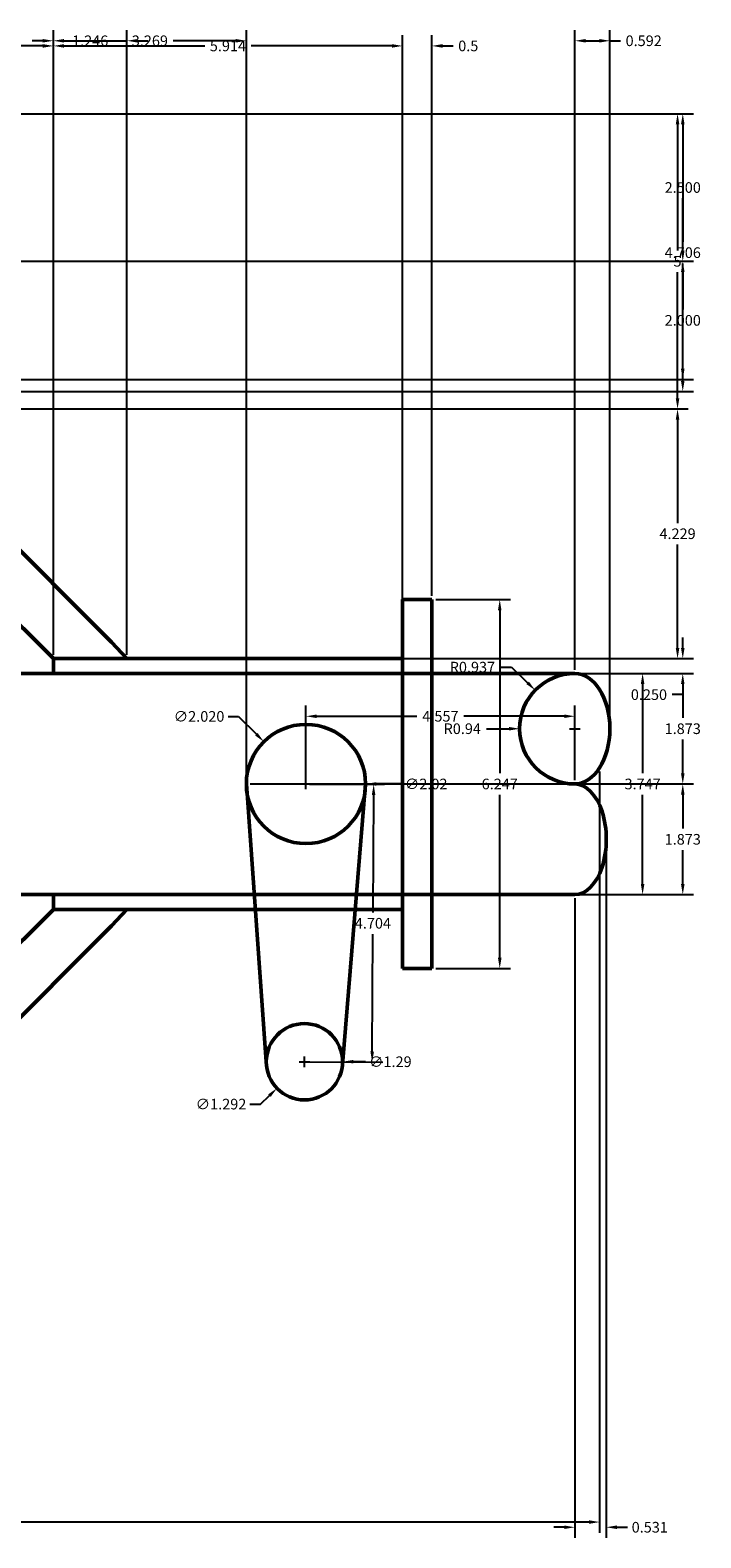
# Model space of a CAD drawing. Units: inches. Extents: x 15.4 to 41.1, y -0.4 to 25.1.
# Tile 4 of 4: x 29.7 to 41.1, y -0.4 to 25.1. Entities that reach past the tile are written whole.
import ezdxf

# ---------------------------------------------------------------- set-up
doc = ezdxf.new("R2010")
doc.units = ezdxf.units.IN
doc.header["$MEASUREMENT"] = 0
doc.layers.add('M-DIMS', color=2, linetype='Continuous', lineweight=18)
doc.layers.add('M-OUTL', color=7, linetype='Continuous', lineweight=50)
doc.styles.get("Standard").update_dxf_attribs({"font": 'arial.ttf'})
doc.dimstyles.get("Standard").update_dxf_attribs({"dimtxt": 0.18, "dimasz": 0.18, "dimexe": 0.18, "dimexo": 0.0625, "dimgap": 0.09, "dimtad": 0, "dimtih": 1, "dimtoh": 1, "dimdec": 4, "dimzin": 0, "dimdsep": 46, "dimtxsty": 'Standard', "dimcen": 0.09, "dimadec": 0, "dimazin": 0, "dimtfac": 1, "dimtdec": 4, "dimtofl": 0, "dimtmove": 0, "dimatfit": 3, "dimfxl": 1, "dimtolj": 1, "dimtzin": 0, "dimarcsym": 0})

# ---------------------------------------------------------------- blocks, each defined once
blk = doc.blocks.new('*D1')
at = {"layer": 'Defpoints', "color": 0, "transparency": 16777216}
for p in [(39.379, 12.649), (17.513, 10.885), (39.379, -0.125)]:
    blk.add_point(p, dxfattribs=at)
at = {"layer": 'M-DIMS', "color": 0, "lineweight": -2, "transparency": 16777216}
for p, q in [((39.379, 12.587), (39.379, -0.305)), ((17.513, 10.823), (17.513, -0.305)), ((17.693, -0.125), (27.98, -0.125)), ((39.199, -0.125), (28.912, -0.125))]:
    blk.add_line(p, q, dxfattribs=at)
at = {"layer": 'M-DIMS', "color": 0, "transparency": 16777216}
for points in [[(17.693, -0.095), (17.693, -0.155), (17.513, -0.125)], [(39.199, -0.095), (39.199, -0.155), (39.379, -0.125)]]:
    blk.add_solid(points, dxfattribs=at)
at = {"layer": 'M-DIMS', "color": 0, "transparency": 16777216, "insert": (28.446, -0.125), "char_height": 0.18, "attachment_point": 5}
blk.add_mtext('\\A1;21.865', dxfattribs=at)
blk = doc.blocks.new('*D8')
at = {"layer": 'Defpoints', "color": 0, "transparency": 16777216}
for p in [(30.124, 24.875), (26.868, 19.021), (30.124, 14.498)]:
    blk.add_point(p, dxfattribs=at)
at = {"layer": 'M-DIMS', "color": 0, "lineweight": -2, "transparency": 16777216}
for p, q in [((26.868, 19.083), (26.868, 25.055)), ((30.124, 14.561), (30.124, 25.055)), ((27.048, 24.875), (28.172, 24.875)), ((29.944, 24.875), (28.819, 24.875))]:
    blk.add_line(p, q, dxfattribs=at)
at = {"layer": 'M-DIMS', "color": 0, "transparency": 16777216}
for points in [[(27.048, 24.905), (27.048, 24.845), (26.868, 24.875)], [(29.944, 24.905), (29.944, 24.845), (30.124, 24.875)]]:
    blk.add_solid(points, dxfattribs=at)
at = {"layer": 'M-DIMS', "color": 0, "transparency": 16777216, "insert": (28.496, 24.875), "char_height": 0.18, "attachment_point": 5}
blk.add_mtext('\\A1;3.26', dxfattribs=at)
blk = doc.blocks.new('*D9')
at = {"layer": 'Defpoints', "color": 0, "transparency": 16777216}
for p in [(36.038, 24.875), (30.124, 14.498), (36.038, 14.498)]:
    blk.add_point(p, dxfattribs=at)
at = {"layer": 'M-DIMS', "color": 0, "lineweight": -2, "transparency": 16777216}
for p, q in [((30.124, 14.561), (30.124, 25.055)), ((36.038, 14.561), (36.038, 25.055)), ((30.304, 24.875), (32.688, 24.875)), ((35.858, 24.875), (33.474, 24.875))]:
    blk.add_line(p, q, dxfattribs=at)
at = {"layer": 'M-DIMS', "color": 0, "transparency": 16777216}
for points in [[(30.304, 24.905), (30.304, 24.845), (30.124, 24.875)], [(35.858, 24.905), (35.858, 24.845), (36.038, 24.875)]]:
    blk.add_solid(points, dxfattribs=at)
at = {"layer": 'M-DIMS', "color": 0, "transparency": 16777216, "insert": (33.081, 24.875), "char_height": 0.18, "attachment_point": 5}
blk.add_mtext('\\A1;5.914', dxfattribs=at)
blk = doc.blocks.new('*D10')
at = {"layer": 'Defpoints', "color": 0, "transparency": 16777216}
for p in [(36.538, 24.875), (36.038, 15.498), (36.538, 15.498)]:
    blk.add_point(p, dxfattribs=at)
at = {"layer": 'M-DIMS', "color": 0, "lineweight": -2, "transparency": 16777216}
for p, q in [((36.038, 15.561), (36.038, 25.055)), ((36.538, 15.561), (36.538, 25.055)), ((35.858, 24.875), (35.678, 24.875)), ((36.718, 24.875), (36.898, 24.875))]:
    blk.add_line(p, q, dxfattribs=at)
at = {"layer": 'M-DIMS', "color": 0, "transparency": 16777216}
for points in [[(35.858, 24.905), (35.858, 24.845), (36.038, 24.875)], [(36.718, 24.905), (36.718, 24.845), (36.538, 24.875)]]:
    blk.add_solid(points, dxfattribs=at)
at = {"layer": 'M-DIMS', "color": 0, "transparency": 16777216, "insert": (37.153, 24.875), "char_height": 0.18, "attachment_point": 5}
blk.add_mtext('\\A1;0.5', dxfattribs=at)
blk = doc.blocks.new('*D11')
at = {"layer": 'Defpoints', "color": 0, "transparency": 16777216}
for p in [(26.868, 23.727), (25.868, 18.727), (40.699, 18.727)]:
    blk.add_point(p, dxfattribs=at)
at = {"layer": 'M-DIMS', "color": 0, "lineweight": -2, "transparency": 16777216}
for p, q in [((26.93, 23.727), (40.879, 23.727)), ((40.699, 23.547), (40.699, 21.409)), ((40.699, 18.907), (40.699, 21.045)), ((25.93, 18.727), (40.879, 18.727))]:
    blk.add_line(p, q, dxfattribs=at)
at = {"layer": 'M-DIMS', "color": 0, "transparency": 16777216}
for points in [[(40.669, 23.547), (40.729, 23.547), (40.699, 23.727)], [(40.669, 18.907), (40.729, 18.907), (40.699, 18.727)]]:
    blk.add_solid(points, dxfattribs=at)
at = {"layer": 'M-DIMS', "color": 0, "transparency": 16777216, "insert": (40.699, 21.227), "char_height": 0.18, "attachment_point": 5}
blk.add_mtext('\\A1;5', dxfattribs=at)
blk = doc.blocks.new('*D12')
at = {"layer": 'Defpoints', "color": 0, "transparency": 16777216}
for p in [(25.868, 18.727), (30.124, 14.498), (40.699, 14.498)]:
    blk.add_point(p, dxfattribs=at)
at = {"layer": 'M-DIMS', "color": 0, "lineweight": -2, "transparency": 16777216}
for p, q in [((25.93, 18.727), (40.879, 18.727)), ((40.699, 18.547), (40.699, 16.794)), ((40.699, 14.678), (40.699, 16.431)), ((30.186, 14.498), (40.879, 14.498))]:
    blk.add_line(p, q, dxfattribs=at)
at = {"layer": 'M-DIMS', "color": 0, "transparency": 16777216}
for points in [[(40.669, 18.547), (40.729, 18.547), (40.699, 18.727)], [(40.669, 14.678), (40.729, 14.678), (40.699, 14.498)]]:
    blk.add_solid(points, dxfattribs=at)
at = {"layer": 'M-DIMS', "color": 0, "transparency": 16777216, "insert": (40.699, 16.613), "char_height": 0.18, "attachment_point": 5}
blk.add_mtext('\\A1;4.229', dxfattribs=at)
blk = doc.blocks.new('*D31')
at = {"layer": 'Defpoints', "color": 0, "transparency": 16777216}
for p in [(38.96, 14.248), (38.96, 10.501), (40.107, 10.501)]:
    blk.add_point(p, dxfattribs=at)
at = {"layer": 'M-DIMS', "color": 0, "lineweight": -2, "transparency": 16777216}
for p, q in [((39.022, 14.248), (40.287, 14.248)), ((40.107, 14.068), (40.107, 12.557)), ((40.107, 10.681), (40.107, 12.193)), ((39.022, 10.501), (40.287, 10.501))]:
    blk.add_line(p, q, dxfattribs=at)
at = {"layer": 'M-DIMS', "color": 0, "transparency": 16777216}
for points in [[(40.077, 14.068), (40.137, 14.068), (40.107, 14.248)], [(40.077, 10.681), (40.137, 10.681), (40.107, 10.501)]]:
    blk.add_solid(points, dxfattribs=at)
at = {"layer": 'M-DIMS', "color": 0, "transparency": 16777216, "insert": (40.107, 12.375), "char_height": 0.18, "attachment_point": 5}
blk.add_mtext('\\A1;3.747', dxfattribs=at)
blk = doc.blocks.new('*D32')
at = {"layer": 'Defpoints', "color": 0, "transparency": 16777216}
for p in [(36.538, 15.498), (36.538, 9.251), (37.686, 9.251)]:
    blk.add_point(p, dxfattribs=at)
at = {"layer": 'M-DIMS', "color": 0, "lineweight": -2, "transparency": 16777216}
for p, q in [((36.601, 15.498), (37.866, 15.498)), ((37.686, 15.318), (37.686, 12.557)), ((37.686, 9.431), (37.686, 12.193)), ((36.601, 9.251), (37.866, 9.251))]:
    blk.add_line(p, q, dxfattribs=at)
at = {"layer": 'M-DIMS', "color": 0, "transparency": 16777216}
for points in [[(37.656, 15.318), (37.716, 15.318), (37.686, 15.498)], [(37.656, 9.431), (37.716, 9.431), (37.686, 9.251)]]:
    blk.add_solid(points, dxfattribs=at)
at = {"layer": 'M-DIMS', "color": 0, "transparency": 16777216, "insert": (37.686, 12.375), "char_height": 0.18, "attachment_point": 5}
blk.add_mtext('\\A1;6.247', dxfattribs=at)
blk = doc.blocks.new('*D33')
at = {"layer": 'Defpoints', "color": 0, "transparency": 16777216}
for p in [(34.403, 12.375), (34.377, 7.671), (35.524, 7.664)]:
    blk.add_point(p, dxfattribs=at)
at = {"layer": 'M-DIMS', "color": 0, "lineweight": -2, "transparency": 16777216}
for p, q in [((34.465, 12.374), (35.73, 12.367)), ((35.549, 12.188), (35.538, 10.198)), ((35.525, 7.844), (35.536, 9.834)), ((34.439, 7.67), (35.704, 7.663))]:
    blk.add_line(p, q, dxfattribs=at)
at = {"layer": 'M-DIMS', "color": 0, "transparency": 16777216}
for points in [[(35.519, 12.189), (35.579, 12.188), (35.55, 12.368)], [(35.495, 7.845), (35.555, 7.844), (35.524, 7.664)]]:
    blk.add_solid(points, dxfattribs=at)
at = {"layer": 'M-DIMS', "color": 0, "transparency": 16777216, "insert": (35.537, 10.016), "char_height": 0.18, "attachment_point": 5}
blk.add_mtext('\\A1;4.704', dxfattribs=at)
blk = doc.blocks.new('*D34')
at = {"layer": 'Defpoints', "color": 0, "transparency": 16777216}
for p in [(38.96, 13.522), (34.403, 12.375), (38.96, 12.375)]:
    blk.add_point(p, dxfattribs=at)
at = {"layer": 'M-DIMS', "color": 0, "lineweight": -2, "transparency": 16777216}
for p, q in [((34.403, 12.437), (34.403, 13.702)), ((38.96, 12.437), (38.96, 13.702)), ((34.583, 13.522), (36.284, 13.522)), ((38.78, 13.522), (37.079, 13.522))]:
    blk.add_line(p, q, dxfattribs=at)
at = {"layer": 'M-DIMS', "color": 0, "transparency": 16777216}
for points in [[(34.583, 13.552), (34.583, 13.492), (34.403, 13.522)], [(38.78, 13.552), (38.78, 13.492), (38.96, 13.522)]]:
    blk.add_solid(points, dxfattribs=at)
at = {"layer": 'M-DIMS', "color": 0, "transparency": 16777216, "insert": (36.681, 13.522), "char_height": 0.18, "attachment_point": 5}
blk.add_mtext('\\A1;4.557', dxfattribs=at)
blk = doc.blocks.new('*D36')
at = {"layer": 'Defpoints', "color": 0, "transparency": 16777216}
for p in [(38.023, 13.311), (38.96, 13.311)]:
    blk.add_point(p, dxfattribs=at)
at = {"layer": 'M-DIMS', "color": 0, "lineweight": -2, "transparency": 16777216}
for p, q in [((37.461, 13.311), (37.843, 13.311)), ((38.87, 13.311), (39.05, 13.311)), ((38.96, 13.221), (38.96, 13.401))]:
    blk.add_line(p, q, dxfattribs=at)
at = {"layer": 'M-DIMS', "color": 0, "transparency": 16777216}
blk.add_solid([(37.843, 13.341), (37.843, 13.281), (38.023, 13.311)], dxfattribs=at)
at = {"layer": 'M-DIMS', "color": 0, "transparency": 16777216, "insert": (37.051, 13.311), "char_height": 0.18, "attachment_point": 5}
blk.add_mtext('\\A1;R0.94', dxfattribs=at)
blk = doc.blocks.new('*D38')
at = {"layer": 'Defpoints', "color": 0, "transparency": 16777216}
for p in [(33.393, 12.374), (35.413, 12.375)]:
    blk.add_point(p, dxfattribs=at)
at = {"layer": 'M-DIMS', "color": 0, "lineweight": -2, "transparency": 16777216}
for p, q in [((34.313, 12.375), (34.493, 12.375)), ((34.403, 12.285), (34.403, 12.465)), ((36.019, 12.375), (35.593, 12.375))]:
    blk.add_line(p, q, dxfattribs=at)
at = {"layer": 'M-DIMS', "color": 0, "transparency": 16777216}
blk.add_solid([(35.593, 12.405), (35.593, 12.345), (35.413, 12.375)], dxfattribs=at)
at = {"layer": 'M-DIMS', "color": 0, "transparency": 16777216, "insert": (36.439, 12.375), "char_height": 0.18, "attachment_point": 5}
blk.add_mtext('\\A1;∅2.02', dxfattribs=at)
blk = doc.blocks.new('*D39')
at = {"layer": 'Defpoints', "color": 0, "transparency": 16777216}
for p in [(33.731, 7.67), (35.023, 7.671)]:
    blk.add_point(p, dxfattribs=at)
at = {"layer": 'M-DIMS', "color": 0, "lineweight": -2, "transparency": 16777216}
for p, q in [((34.287, 7.671), (34.467, 7.671)), ((34.377, 7.581), (34.377, 7.761)), ((35.41, 7.671), (35.203, 7.671))]:
    blk.add_line(p, q, dxfattribs=at)
at = {"layer": 'M-DIMS', "color": 0, "transparency": 16777216}
blk.add_solid([(35.203, 7.701), (35.203, 7.641), (35.023, 7.671)], dxfattribs=at)
at = {"layer": 'M-DIMS', "color": 0, "transparency": 16777216, "insert": (35.832, 7.671), "char_height": 0.18, "attachment_point": 5}
blk.add_mtext('\\A1;∅1.29', dxfattribs=at)
blk = doc.blocks.new('*D43')
at = {"layer": 'Defpoints', "color": 0, "transparency": 16777216}
for p in [(23.368, 23.727), (23.368, 21.227), (40.787, 21.227)]:
    blk.add_point(p, dxfattribs=at)
at = {"layer": 'M-DIMS', "color": 0, "lineweight": -2, "transparency": 16777216}
for p, q in [((23.43, 23.727), (40.967, 23.727)), ((40.787, 23.547), (40.787, 22.659)), ((40.787, 21.407), (40.787, 22.295)), ((23.43, 21.227), (40.967, 21.227))]:
    blk.add_line(p, q, dxfattribs=at)
at = {"layer": 'M-DIMS', "color": 0, "transparency": 16777216}
for points in [[(40.757, 23.547), (40.817, 23.547), (40.787, 23.727)], [(40.757, 21.407), (40.817, 21.407), (40.787, 21.227)]]:
    blk.add_solid(points, dxfattribs=at)
at = {"layer": 'M-DIMS', "color": 0, "transparency": 16777216, "insert": (40.787, 22.477), "char_height": 0.18, "attachment_point": 5}
blk.add_mtext('\\A1;2.500', dxfattribs=at)
blk = doc.blocks.new('*D44')
at = {"layer": 'Defpoints', "color": 0, "transparency": 16777216}
for p in [(25.868, 21.227), (25.868, 19.227), (40.787, 19.227)]:
    blk.add_point(p, dxfattribs=at)
at = {"layer": 'M-DIMS', "color": 0, "lineweight": -2, "transparency": 16777216}
for p, q in [((25.93, 21.227), (40.967, 21.227)), ((40.787, 21.047), (40.787, 20.409)), ((40.787, 19.407), (40.787, 20.045)), ((25.93, 19.227), (40.967, 19.227))]:
    blk.add_line(p, q, dxfattribs=at)
at = {"layer": 'M-DIMS', "color": 0, "transparency": 16777216}
for points in [[(40.757, 21.047), (40.817, 21.047), (40.787, 21.227)], [(40.757, 19.407), (40.817, 19.407), (40.787, 19.227)]]:
    blk.add_solid(points, dxfattribs=at)
at = {"layer": 'M-DIMS', "color": 0, "transparency": 16777216, "insert": (40.787, 20.227), "char_height": 0.18, "attachment_point": 5}
blk.add_mtext('\\A1;2.000', dxfattribs=at)
blk = doc.blocks.new('*D45')
at = {"layer": 'Defpoints', "color": 0, "transparency": 16777216}
for p in [(31.37, 24.962), (30.124, 14.498), (31.37, 14.498)]:
    blk.add_point(p, dxfattribs=at)
at = {"layer": 'M-DIMS', "color": 0, "lineweight": -2, "transparency": 16777216}
for p, q in [((30.124, 14.561), (30.124, 25.142)), ((31.37, 14.561), (31.37, 25.142)), ((29.944, 24.962), (29.764, 24.962)), ((31.55, 24.962), (31.73, 24.962))]:
    blk.add_line(p, q, dxfattribs=at)
at = {"layer": 'M-DIMS', "color": 0, "transparency": 16777216}
for points in [[(29.944, 24.992), (29.944, 24.932), (30.124, 24.962)], [(31.55, 24.992), (31.55, 24.932), (31.37, 24.962)]]:
    blk.add_solid(points, dxfattribs=at)
at = {"layer": 'M-DIMS', "color": 0, "transparency": 16777216, "insert": (30.747, 24.962), "char_height": 0.18, "attachment_point": 5}
blk.add_mtext('\\A1;1.246', dxfattribs=at)
blk = doc.blocks.new('*D46')
at = {"layer": 'Defpoints', "color": 0, "transparency": 16777216}
for p in [(26.868, 23.727), (26.868, 19.021), (40.787, 19.021)]:
    blk.add_point(p, dxfattribs=at)
at = {"layer": 'M-DIMS', "color": 0, "lineweight": -2, "transparency": 16777216}
for p, q in [((26.93, 23.727), (40.967, 23.727)), ((40.787, 23.547), (40.787, 21.556)), ((40.787, 19.201), (40.787, 21.192)), ((26.93, 19.021), (40.967, 19.021))]:
    blk.add_line(p, q, dxfattribs=at)
at = {"layer": 'M-DIMS', "color": 0, "transparency": 16777216}
for points in [[(40.757, 23.547), (40.817, 23.547), (40.787, 23.727)], [(40.757, 19.201), (40.817, 19.201), (40.787, 19.021)]]:
    blk.add_solid(points, dxfattribs=at)
at = {"layer": 'M-DIMS', "color": 0, "transparency": 16777216, "insert": (40.787, 21.374), "char_height": 0.18, "attachment_point": 5}
blk.add_mtext('\\A1;4.706', dxfattribs=at)
blk = doc.blocks.new('*D47')
at = {"layer": 'Defpoints', "color": 0, "transparency": 16777216}
for p in [(30.124, 14.498), (30.124, 14.248), (40.787, 14.248)]:
    blk.add_point(p, dxfattribs=at)
at = {"layer": 'M-DIMS', "color": 0, "lineweight": -2, "transparency": 16777216}
for p, q in [((40.787, 14.678), (40.787, 14.858)), ((30.186, 14.498), (40.967, 14.498)), ((30.186, 14.248), (40.967, 14.248)), ((40.787, 14.068), (40.787, 13.888)), ((40.787, 13.888), (40.607, 13.888))]:
    blk.add_line(p, q, dxfattribs=at)
at = {"layer": 'M-DIMS', "color": 0, "transparency": 16777216}
for points in [[(40.757, 14.678), (40.817, 14.678), (40.787, 14.498)], [(40.757, 14.068), (40.817, 14.068), (40.787, 14.248)]]:
    blk.add_solid(points, dxfattribs=at)
at = {"layer": 'M-DIMS', "color": 0, "transparency": 16777216, "insert": (40.214, 13.888), "char_height": 0.18, "attachment_point": 5}
blk.add_mtext('\\A1;0.250', dxfattribs=at)
blk = doc.blocks.new('*D48')
at = {"layer": 'Defpoints', "color": 0, "transparency": 16777216}
for p in [(33.393, 24.962), (30.124, 14.498), (33.393, 12.375)]:
    blk.add_point(p, dxfattribs=at)
at = {"layer": 'M-DIMS', "color": 0, "lineweight": -2, "transparency": 16777216}
for p, q in [((30.124, 14.561), (30.124, 25.142)), ((33.393, 12.437), (33.393, 25.142)), ((30.304, 24.962), (31.364, 24.962)), ((33.213, 24.962), (32.152, 24.962))]:
    blk.add_line(p, q, dxfattribs=at)
at = {"layer": 'M-DIMS', "color": 0, "transparency": 16777216}
for points in [[(30.304, 24.992), (30.304, 24.932), (30.124, 24.962)], [(33.213, 24.992), (33.213, 24.932), (33.393, 24.962)]]:
    blk.add_solid(points, dxfattribs=at)
at = {"layer": 'M-DIMS', "color": 0, "transparency": 16777216, "insert": (31.758, 24.962), "char_height": 0.18, "attachment_point": 5}
blk.add_mtext('\\A1;3.269', dxfattribs=at)
blk = doc.blocks.new('*D49')
at = {"layer": 'Defpoints', "color": 0, "transparency": 16777216}
for p in [(33.393, 12.375), (40.787, 12.375), (30.124, 10.501)]:
    blk.add_point(p, dxfattribs=at)
at = {"layer": 'M-DIMS', "color": 0, "lineweight": -2, "transparency": 16777216}
for p, q in [((33.455, 12.375), (40.967, 12.375)), ((40.787, 12.195), (40.787, 11.62)), ((40.787, 10.681), (40.787, 11.256)), ((30.186, 10.501), (40.967, 10.501))]:
    blk.add_line(p, q, dxfattribs=at)
at = {"layer": 'M-DIMS', "color": 0, "transparency": 16777216}
for points in [[(40.757, 12.195), (40.817, 12.195), (40.787, 12.375)], [(40.757, 10.681), (40.817, 10.681), (40.787, 10.501)]]:
    blk.add_solid(points, dxfattribs=at)
at = {"layer": 'M-DIMS', "color": 0, "transparency": 16777216, "insert": (40.787, 11.438), "char_height": 0.18, "attachment_point": 5}
blk.add_mtext('\\A1;1.873', dxfattribs=at)
blk = doc.blocks.new('*D52')
at = {"layer": 'Defpoints', "color": 0, "transparency": 16777216}
for p in [(39.552, 24.962), (38.96, 14.248), (39.552, 13.311)]:
    blk.add_point(p, dxfattribs=at)
at = {"layer": 'M-DIMS', "color": 0, "lineweight": -2, "transparency": 16777216}
for p, q in [((38.96, 14.311), (38.96, 25.142)), ((39.552, 13.374), (39.552, 25.142)), ((39.14, 24.962), (39.372, 24.962)), ((39.552, 24.962), (39.732, 24.962))]:
    blk.add_line(p, q, dxfattribs=at)
at = {"layer": 'M-DIMS', "color": 0, "transparency": 16777216}
for points in [[(39.14, 24.992), (39.14, 24.932), (38.96, 24.962)], [(39.372, 24.992), (39.372, 24.932), (39.552, 24.962)]]:
    blk.add_solid(points, dxfattribs=at)
at = {"layer": 'M-DIMS', "color": 0, "transparency": 16777216, "insert": (40.125, 24.962), "char_height": 0.18, "attachment_point": 5}
blk.add_mtext('\\A1;0.592', dxfattribs=at)
blk = doc.blocks.new('*D53')
at = {"layer": 'Defpoints', "color": 0, "transparency": 16777216}
for p in [(39.491, 11.438), (38.96, 10.501), (39.491, -0.213)]:
    blk.add_point(p, dxfattribs=at)
at = {"layer": 'M-DIMS', "color": 0, "lineweight": -2, "transparency": 16777216}
for p, q in [((39.491, 11.375), (39.491, -0.393)), ((38.96, 10.439), (38.96, -0.393)), ((38.78, -0.213), (38.6, -0.213)), ((39.671, -0.213), (39.851, -0.213))]:
    blk.add_line(p, q, dxfattribs=at)
at = {"layer": 'M-DIMS', "color": 0, "transparency": 16777216}
for points in [[(38.78, -0.183), (38.78, -0.243), (38.96, -0.213)], [(39.671, -0.183), (39.671, -0.243), (39.491, -0.213)]]:
    blk.add_solid(points, dxfattribs=at)
at = {"layer": 'M-DIMS', "color": 0, "transparency": 16777216, "insert": (40.228, -0.213), "char_height": 0.18, "attachment_point": 5}
blk.add_mtext('\\A1;0.531', dxfattribs=at)
blk = doc.blocks.new('*D54')
at = {"layer": 'Defpoints', "color": 0, "transparency": 16777216}
for p in [(38.96, 14.248), (38.96, 12.375), (40.787, 12.375)]:
    blk.add_point(p, dxfattribs=at)
at = {"layer": 'M-DIMS', "color": 0, "lineweight": -2, "transparency": 16777216}
for p, q in [((39.022, 14.248), (40.967, 14.248)), ((40.787, 14.068), (40.787, 13.493)), ((40.787, 12.555), (40.787, 13.129)), ((39.022, 12.375), (40.967, 12.375))]:
    blk.add_line(p, q, dxfattribs=at)
at = {"layer": 'M-DIMS', "color": 0, "transparency": 16777216}
for points in [[(40.757, 14.068), (40.817, 14.068), (40.787, 14.248)], [(40.757, 12.555), (40.817, 12.555), (40.787, 12.375)]]:
    blk.add_solid(points, dxfattribs=at)
at = {"layer": 'M-DIMS', "color": 0, "transparency": 16777216, "insert": (40.787, 13.311), "char_height": 0.18, "attachment_point": 5}
blk.add_mtext('\\A1;1.873', dxfattribs=at)
blk = doc.blocks.new('*D56')
at = {"layer": 'Defpoints', "color": 0, "transparency": 16777216}
for p in [(38.287, 13.963), (38.96, 13.311)]:
    blk.add_point(p, dxfattribs=at)
at = {"layer": 'M-DIMS', "color": 0, "lineweight": -2, "transparency": 16777216}
for p, q in [((37.703, 14.354), (37.883, 14.354)), ((37.883, 14.354), (38.158, 14.088)), ((38.87, 13.311), (39.05, 13.311)), ((38.96, 13.221), (38.96, 13.401))]:
    blk.add_line(p, q, dxfattribs=at)
at = {"layer": 'M-DIMS', "color": 0, "transparency": 16777216}
blk.add_solid([(38.179, 14.11), (38.137, 14.067), (38.287, 13.963)], dxfattribs=at)
at = {"layer": 'M-DIMS', "color": 0, "transparency": 16777216, "insert": (37.223, 14.354), "char_height": 0.18, "attachment_point": 5}
blk.add_mtext('\\A1;R0.937', dxfattribs=at)
blk = doc.blocks.new('*D58')
at = {"layer": 'Defpoints', "color": 0, "transparency": 16777216}
for p in [(33.69, 13.09), (35.116, 11.659)]:
    blk.add_point(p, dxfattribs=at)
at = {"layer": 'M-DIMS', "color": 0, "lineweight": -2, "transparency": 16777216}
for p, q in [((33.082, 13.519), (33.262, 13.519)), ((33.262, 13.519), (33.563, 13.218)), ((34.313, 12.375), (34.493, 12.375)), ((34.403, 12.285), (34.403, 12.465))]:
    blk.add_line(p, q, dxfattribs=at)
at = {"layer": 'M-DIMS', "color": 0, "transparency": 16777216}
blk.add_solid([(33.584, 13.239), (33.541, 13.197), (33.69, 13.09)], dxfattribs=at)
at = {"layer": 'M-DIMS', "color": 0, "transparency": 16777216, "insert": (32.591, 13.519), "char_height": 0.18, "attachment_point": 5}
blk.add_mtext('\\A1;∅2.020', dxfattribs=at)
blk = doc.blocks.new('*D59')
at = {"layer": 'Defpoints', "color": 0, "transparency": 16777216}
for p in [(34.841, 8.119), (33.912, 7.222)]:
    blk.add_point(p, dxfattribs=at)
at = {"layer": 'M-DIMS', "color": 0, "lineweight": -2, "transparency": 16777216}
for p, q in [((34.287, 7.671), (34.467, 7.671)), ((34.377, 7.581), (34.377, 7.761)), ((33.454, 6.953), (33.634, 6.953)), ((33.634, 6.953), (33.783, 7.097))]:
    blk.add_line(p, q, dxfattribs=at)
at = {"layer": 'M-DIMS', "color": 0, "transparency": 16777216}
blk.add_solid([(33.762, 7.118), (33.804, 7.075), (33.912, 7.222)], dxfattribs=at)
at = {"layer": 'M-DIMS', "color": 0, "transparency": 16777216, "insert": (32.963, 6.953), "char_height": 0.18, "attachment_point": 5}
blk.add_mtext('\\A1;∅1.292', dxfattribs=at)

msp = doc.modelspace()

# ---------------------------------------------------------------- linework, layer by layer
at = {"layer": 'M-OUTL'}
for p, q in [((26.8676, 19.0206), (31.1089, 14.7766)), ((25.8676, 18.727), (30.124, 14.4982)), ((36.038, 14.4982), (36.038, 15.4982)), ((36.038, 15.4982), (36.538, 15.4982)), ((36.538, 15.4982), (36.538, 9.2512)), ((31.1089, 14.7766), (31.3702, 14.4982)), ((30.124, 14.4982), (36.038, 14.4982)), ((30.124, 14.4982), (30.124, 14.2482)), ((36.038, 14.4982), (36.038, 10.2512)), ((30.124, 14.2482), (24.374, 14.2482)), ((30.124, 14.2482), (37.9598, 14.2482)), ((37.9598, 14.2482), (38.9598, 14.2482)), ((33.3927, 12.3747), (33.731, 7.6707)), ((35.4126, 12.3747), (35.0204, 7.6176)), ((30.124, 10.5012), (24.374, 10.5012)), ((30.124, 10.5012), (24.374, 10.5012)), ((30.124, 10.2512), (30.124, 10.5012)), ((30.124, 10.5012), (37.9598, 10.5012)), ((30.124, 10.2512), (30.124, 10.5012)), ((30.124, 10.5012), (37.9598, 10.5012)), ((37.9598, 10.5012), (38.9598, 10.5012)), ((25.8676, 6.0224), (30.124, 10.2512)), ((25.8676, 6.0224), (30.124, 10.2512)), ((30.124, 10.2512), (36.038, 10.2512)), ((30.124, 10.2512), (36.038, 10.2512)), ((31.1089, 9.9728), (31.3702, 10.2512)), ((31.1089, 9.9728), (31.3702, 10.2512)), ((36.038, 10.2512), (36.038, 9.2512)), ((26.8676, 5.7288), (31.1089, 9.9728)), ((26.8676, 5.7288), (31.1089, 9.9728)), ((36.038, 9.2512), (36.538, 9.2512))]:
    msp.add_line(p, q, dxfattribs=at)
for centre, radius in [((34.4026, 12.3747), 1.01), ((34.3768, 7.6707), 0.6458)]:
    msp.add_circle(centre, radius, dxfattribs=at)
msp.add_arc((38.9598, 13.3114), 0.9367, 90, 270, dxfattribs=at)
for centre, major_axis, ratio, start_param, end_param in [((38.9598, 13.3114), (0, 0.9367), 0.6321648, 3.1415927, 6.2831853), ((38.9598, 11.438), (0, -0.9367), 0.5673736, 0, 3.1415927)]:
    msp.add_ellipse(centre, major_axis=major_axis, ratio=ratio, start_param=start_param, end_param=end_param, dxfattribs=at)

# ---------------------------------------------------------------- dimensions: what is measured, and where the dimension line sits
at = {"layer": 'M-DIMS'}
for base, p1, p2, override, picture, middle in [((30.124, 24.8745), (26.8676, 19.0206), (30.124, 14.4982), {"dimdec": 2, "dimlfac": 1, "dimrnd": 0, "dimzin": 0, "dimdsep": 46, "dimlunit": 2}, '*D8', (28.4958, 24.8745)), ((31.3702, 24.962), (30.124, 14.4982), (31.3702, 14.4982), {"dimdec": 3, "dimlfac": 1, "dimrnd": 0, "dimzin": 0, "dimdsep": 46, "dimlunit": 2}, '*D45', (30.7471, 24.962)), ((33.3927, 24.962), (30.124, 14.4982), (33.3927, 12.3747), {"dimdec": 3, "dimlfac": 1, "dimrnd": 0, "dimzin": 0, "dimdsep": 46, "dimlunit": 2}, '*D48', (31.7583, 24.962)), ((36.038, 24.8745), (30.124, 14.4982), (36.038, 14.4982), {"dimdec": 3, "dimlfac": 1, "dimrnd": 0, "dimzin": 0, "dimdsep": 46, "dimlunit": 2}, '*D9', (33.081, 24.8745)), ((36.538, 24.8745), (36.038, 15.4982), (36.538, 15.4982), {"dimdec": 1, "dimlfac": 1, "dimrnd": 0, "dimzin": 0, "dimdsep": 46, "dimlunit": 2}, '*D10', (37.1525, 24.8745)), ((39.552, 24.962), (38.9598, 14.2482), (39.552, 13.3114), {"dimdec": 3, "dimlfac": 1, "dimrnd": 0, "dimzin": 0, "dimdsep": 46, "dimlunit": 2}, '*D52', (40.1247, 24.962)), ((38.9598, 13.5222), (34.4026, 12.3747), (38.9598, 12.3747), {"dimdec": 3, "dimlfac": 1, "dimrnd": 0, "dimzin": 0, "dimdsep": 46, "dimlunit": 2}, '*D34', (36.6812, 13.5222)), ((39.3785, -0.1251), (17.5132, 10.8851), (39.3785, 12.6491), {"dimdec": 3, "dimlfac": 1, "dimrnd": 0, "dimzin": 0, "dimdsep": 46, "dimlunit": 2}, '*D1', (28.4458, -0.1251)), ((39.49126, -0.21262), (38.95978, 10.50123), (39.49126, 11.43796), {"dimdec": 3, "dimlfac": 1, "dimrnd": 0, "dimzin": 0, "dimdsep": 46, "dimlunit": 2}, '*D53', (40.22759, -0.21262))]:
    dim = msp.add_linear_dim(base=base, p1=p1, p2=p2, dimstyle='Standard', override=override, dxfattribs=at)
    dim.commit()
    dim.dimension.update_dxf_attribs({"geometry": picture, "text_midpoint": middle})
for base, p1, p2, angle, override, picture, middle in [((40.787, 21.227), (23.3676, 23.727), (23.3676, 21.227), 90, {"dimdec": 3, "dimlfac": 1, "dimrnd": 0, "dimzin": 0, "dimdsep": 46, "dimlunit": 2}, '*D43', (40.787, 22.477)), ((40.6995, 18.727), (26.8676, 23.727), (25.8676, 18.727), 90, {"dimdec": 0, "dimlfac": 1, "dimrnd": 0, "dimzin": 0, "dimdsep": 46, "dimlunit": 2}, '*D11', (40.6995, 21.227)), ((40.787, 19.0206), (26.8676, 23.727), (26.8676, 19.0206), 90, {"dimdec": 3, "dimlfac": 1, "dimrnd": 0, "dimzin": 0, "dimdsep": 46, "dimlunit": 2}, '*D46', (40.787, 21.3738)), ((40.787, 19.227), (25.8676, 21.227), (25.8676, 19.227), 90, {"dimdec": 3, "dimlfac": 1, "dimrnd": 0, "dimzin": 0, "dimdsep": 46, "dimlunit": 2}, '*D44', (40.787, 20.227)), ((40.6995, 14.4982), (25.8676, 18.727), (30.124, 14.4982), 90, {"dimdec": 3, "dimlfac": 1, "dimrnd": 0, "dimzin": 0, "dimdsep": 46, "dimlunit": 2}, '*D12', (40.6995, 16.6126)), ((37.6855, 9.2512), (36.538, 15.4982), (36.538, 9.2512), 270, {"dimdec": 3, "dimlfac": 1, "dimrnd": 0, "dimzin": 0, "dimdsep": 46, "dimlunit": 2}, '*D32', (37.6855, 12.3747)), ((40.787, 14.2482), (30.124, 14.4982), (30.124, 14.2482), 90, {"dimdec": 3, "dimlfac": 1, "dimrnd": 0, "dimzin": 0, "dimdsep": 46, "dimlunit": 2}, '*D47', (40.2136, 13.8882)), ((40.1073, 10.5012), (38.9598, 14.2482), (38.9598, 10.5012), 270, {"dimdec": 3, "dimlfac": 1, "dimrnd": 0, "dimzin": 0, "dimdsep": 46, "dimlunit": 2}, '*D31', (40.1073, 12.3747)), ((40.78695, 12.37469), (38.95978, 14.24816), (38.95978, 12.37469), 90, {"dimdec": 3, "dimlfac": 1, "dimrnd": 0, "dimzin": 0, "dimdsep": 46, "dimlunit": 2}, '*D54', (40.78695, 13.31143)), ((40.78695, 12.3747), (30.12396, 10.50123), (33.39267, 12.37469), 90, {"dimdec": 3, "dimlfac": 1, "dimrnd": 0, "dimzin": 0, "dimdsep": 46, "dimlunit": 2}, '*D49', (40.78695, 11.43796)), ((35.5243, 7.6644), (34.4026, 12.3747), (34.3768, 7.6707), 269.68489, {"dimdec": 3, "dimlfac": 1, "dimrnd": 0, "dimzin": 0, "dimdsep": 46, "dimlunit": 2}, '*D33', (35.5372, 10.0164))]:
    dim = msp.add_linear_dim(base=base, p1=p1, p2=p2, angle=angle, dimstyle='Standard', override=override, dxfattribs=at)
    dim.commit()
    dim.dimension.update_dxf_attribs({"geometry": picture, "text_midpoint": middle})
for mpoint, override, picture, middle in [((38.287, 13.9632), {"dimdec": 3, "dimlfac": 1, "dimrnd": 0, "dimzin": 0, "dimdsep": 46, "dimlunit": 2}, '*D56', (37.2235, 14.3543)), ((38.0231, 13.311), {"dimdec": 2, "dimlfac": 1, "dimrnd": 0, "dimzin": 0, "dimdsep": 46, "dimlunit": 2}, '*D36', (37.461, 13.3107))]:
    dim = msp.add_radius_dim(center=(38.9598, 13.3114), mpoint=mpoint, dimstyle='Standard', override=override, dxfattribs=at)
    dim.commit()
    dim.dimension.update_dxf_attribs({"geometry": picture, "text_midpoint": middle, "dimtype": 164})
for p1, p2, override, picture, middle in [((35.1155, 11.6592), (33.6898, 13.0902), {"dimdec": 3, "dimlfac": 1, "dimrnd": 0, "dimzin": 0, "dimdsep": 46, "dimlunit": 2}, '*D58', (32.5908, 13.5195)), ((33.3927, 12.3744), (35.4126, 12.375), {"dimdec": 2, "dimlfac": 1, "dimrnd": 0, "dimzin": 0, "dimdsep": 46, "dimlunit": 2}, '*D38', (36.0186, 12.3752)), ((34.8412, 8.1194), (33.9124, 7.2219), {"dimdec": 3, "dimlfac": 1, "dimrnd": 0, "dimzin": 0, "dimdsep": 46, "dimlunit": 2}, '*D59', (32.963, 6.9527)), ((33.731, 7.6703), (35.0226, 7.671), {"dimdec": 2, "dimlfac": 1, "dimrnd": 0, "dimzin": 0, "dimdsep": 46, "dimlunit": 2}, '*D39', (35.41, 7.6712))]:
    dim = msp.add_diameter_dim_2p(p1=p1, p2=p2, dimstyle='Standard', override=override, dxfattribs=at)
    dim.commit()
    dim.dimension.update_dxf_attribs({"geometry": picture, "text_midpoint": middle, "dimtype": 163})

doc.saveas('drawing.dxf')
